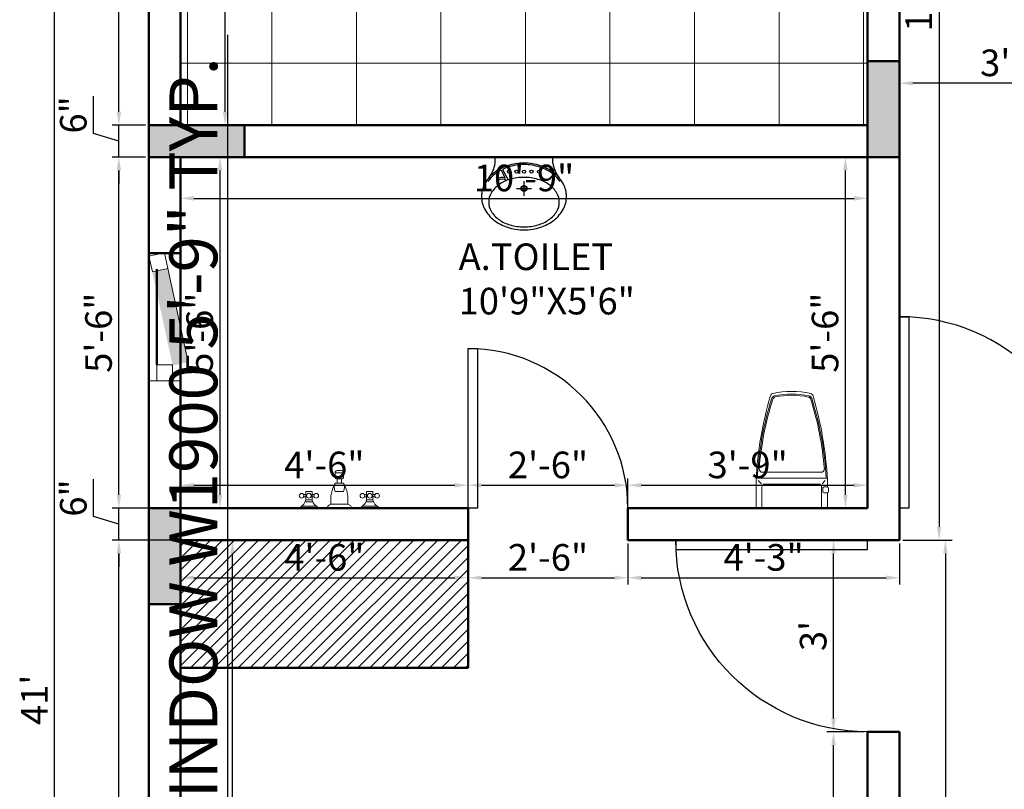
# Model space of a CAD drawing. Units: inches. Extents: x 3064 to 19385, y 846 to 15425.
# Tile 100 of 108: x 7502 to 7687, y 1134 to 1278. Entities that reach past the tile are written whole.
import ezdxf

# ---------------------------------------------------------------- set-up
doc = ezdxf.new("R2010")
doc.units = ezdxf.units.IN
for name, color, linetype, lineweight in [('A-ANNO-DIMS', 2, 'Continuous', 18), ('A-AREA-IDEN', 3, 'Continuous', 18), ('A-COLS', 1, 'Continuous', 35), ('A-DOOR', 3, 'Continuous', 25), ('A-FLOR-FIXT', 9, 'Continuous', 18), ('A-FLOR-PATT', 252, 'Continuous', 13), ('A-FURN-PATT', 252, 'Continuous', 13), ('A-GLAZ', 4, 'Continuous', 18), ('A-WALL', 7, 'Continuous', 50)]:
    doc.layers.add(name, color=color, linetype=linetype, lineweight=lineweight)
doc.layers.add('THIET-BI', color=21, linetype='Continuous')
doc.styles.get("Standard").update_dxf_attribs({"font": 'arial.ttf'})
doc.dimstyles.new('ISO-25', dxfattribs={"dimtxt": 9, "dimasz": 2.5, "dimexe": 1.25, "dimexo": 0.625, "dimtad": 1, "dimdec": 1, "dimlunit": 3, "dimtxsty": 'Standard', "dimcen": 2.5, "dimadec": 0, "dimazin": 0, "dimtfac": 1, "dimtdec": 1, "dimtmove": 0, "dimatfit": 3, "dimfxl": 1, "dimarcsym": 0})

# ---------------------------------------------------------------- blocks, each defined once
blk = doc.blocks.new('*U3')
for p, q in [((0, 0), (0, -6)), ((36, 0), (36, -6))]:
    blk.add_line(p, q)
blk.add_lwpolyline([(0, 0), (0, 36), (1.75, 36), (1.75, 0)], close=True)
blk.add_arc((0, 0), 36, 0, 90)
blk = doc.blocks.new('*U4')
for p, q in [((0, 0), (0, -6)), ((30, 0), (30, -6))]:
    blk.add_line(p, q)
blk.add_lwpolyline([(0, 0), (0, 30), (1.75, 30), (1.75, 0)], close=True)
blk.add_arc((0, 0), 30, 0, 90)
blk = doc.blocks.new('*D318')
at = {"layer": 'A-ANNO-DIMS', "color": 0, "lineweight": -2, "transparency": 16777216}
for p, q in [((7531.62, 1180.34), (7519.4, 1180.34)), ((7520.65, 984.84), (7520.65, 1177.84)), ((7531.62, 982.34), (7519.4, 982.34))]:
    blk.add_line(p, q, dxfattribs=at)
at = {"layer": 'A-ANNO-DIMS', "color": 0, "transparency": 16777216}
for points in [[(7520.23, 1177.84), (7521.06, 1177.84), (7520.65, 1180.34)], [(7520.23, 984.84), (7521.06, 984.84), (7520.65, 982.34)]]:
    blk.add_solid(points, dxfattribs=at)
at = {"layer": 'Defpoints', "color": 0, "transparency": 16777216}
for p in [(7520.65, 1180.34), (7532.25, 1180.34), (7532.25, 982.34)]:
    blk.add_point(p, dxfattribs=at)
at = {"layer": 'A-ANNO-DIMS', "color": 0, "transparency": 16777216, "insert": (7517.47, 1081.34), "char_height": 5, "attachment_point": 5, "rotation": 90}
blk.add_mtext('16\'-6"', dxfattribs=at)
blk = doc.blocks.new('*D319')
at = {"layer": 'A-ANNO-DIMS', "color": 0, "lineweight": -2, "transparency": 16777216}
for p, q in [((7515.91, 1184.76), (7515.91, 1191.79)), ((7520.65, 1188.84), (7520.65, 1191.34)), ((7531.62, 1186.34), (7519.4, 1186.34)), ((7520.65, 1180.34), (7520.65, 1186.34)), ((7520.65, 1180.34), (7520.65, 1186.34)), ((7520.65, 1183.34), (7515.91, 1184.76)), ((7531.62, 1180.34), (7519.4, 1180.34)), ((7520.65, 1177.84), (7520.65, 1175.34))]:
    blk.add_line(p, q, dxfattribs=at)
at = {"layer": 'A-ANNO-DIMS', "color": 0, "transparency": 16777216}
for points in [[(7520.23, 1188.84), (7521.06, 1188.84), (7520.65, 1186.34)], [(7520.23, 1177.84), (7521.06, 1177.84), (7520.65, 1180.34)]]:
    blk.add_solid(points, dxfattribs=at)
at = {"layer": 'Defpoints', "color": 0, "transparency": 16777216}
for p in [(7520.65, 1186.34), (7532.25, 1186.34), (7532.25, 1180.34)]:
    blk.add_point(p, dxfattribs=at)
at = {"layer": 'A-ANNO-DIMS', "color": 0, "transparency": 16777216, "insert": (7512.73, 1188.27), "char_height": 5, "attachment_point": 5, "rotation": 90}
blk.add_mtext('6"', dxfattribs=at)
blk = doc.blocks.new('*D320')
at = {"layer": 'A-ANNO-DIMS', "color": 0, "lineweight": -2, "transparency": 16777216}
for p, q in [((7525.62, 1252.34), (7519.4, 1252.34)), ((7520.65, 1188.84), (7520.65, 1249.84)), ((7531.62, 1186.34), (7519.4, 1186.34))]:
    blk.add_line(p, q, dxfattribs=at)
at = {"layer": 'A-ANNO-DIMS', "color": 0, "transparency": 16777216}
for points in [[(7520.23, 1249.84), (7521.06, 1249.84), (7520.65, 1252.34)], [(7520.23, 1188.84), (7521.06, 1188.84), (7520.65, 1186.34)]]:
    blk.add_solid(points, dxfattribs=at)
at = {"layer": 'Defpoints', "color": 0, "transparency": 16777216}
for p in [(7520.65, 1252.34), (7526.25, 1252.34), (7532.25, 1186.34)]:
    blk.add_point(p, dxfattribs=at)
at = {"layer": 'A-ANNO-DIMS', "color": 0, "transparency": 16777216, "insert": (7517.47, 1219.34), "char_height": 5, "attachment_point": 5, "rotation": 90}
blk.add_mtext('5\'-6"', dxfattribs=at)
blk = doc.blocks.new('*D321')
at = {"layer": 'A-ANNO-DIMS', "color": 0, "lineweight": -2, "transparency": 16777216}
for p, q in [((7515.91, 1256.76), (7515.91, 1263.79)), ((7520.65, 1260.84), (7520.65, 1263.34)), ((7525.62, 1258.34), (7519.4, 1258.34)), ((7520.65, 1252.34), (7520.65, 1258.34)), ((7520.65, 1252.34), (7520.65, 1258.34)), ((7520.65, 1255.34), (7515.91, 1256.76)), ((7525.62, 1252.34), (7519.4, 1252.34)), ((7520.65, 1249.84), (7520.65, 1247.34))]:
    blk.add_line(p, q, dxfattribs=at)
at = {"layer": 'A-ANNO-DIMS', "color": 0, "transparency": 16777216}
for points in [[(7520.23, 1260.84), (7521.06, 1260.84), (7520.65, 1258.34)], [(7520.23, 1249.84), (7521.06, 1249.84), (7520.65, 1252.34)]]:
    blk.add_solid(points, dxfattribs=at)
at = {"layer": 'Defpoints', "color": 0, "transparency": 16777216}
for p in [(7520.65, 1258.34), (7526.25, 1258.34), (7526.25, 1252.34)]:
    blk.add_point(p, dxfattribs=at)
at = {"layer": 'A-ANNO-DIMS', "color": 0, "transparency": 16777216, "insert": (7512.73, 1260.27), "char_height": 5, "attachment_point": 5, "rotation": 90}
blk.add_mtext('6"', dxfattribs=at)
blk = doc.blocks.new('*D322')
at = {"layer": 'A-ANNO-DIMS', "color": 0, "lineweight": -2, "transparency": 16777216}
for p, q in [((7531.62, 1390.34), (7519.4, 1390.34)), ((7520.65, 1260.84), (7520.65, 1387.84)), ((7525.62, 1258.34), (7519.4, 1258.34))]:
    blk.add_line(p, q, dxfattribs=at)
at = {"layer": 'A-ANNO-DIMS', "color": 0, "transparency": 16777216}
for points in [[(7520.23, 1387.84), (7521.06, 1387.84), (7520.65, 1390.34)], [(7520.23, 1260.84), (7521.06, 1260.84), (7520.65, 1258.34)]]:
    blk.add_solid(points, dxfattribs=at)
at = {"layer": 'Defpoints', "color": 0, "transparency": 16777216}
for p in [(7520.65, 1390.34), (7532.25, 1390.34), (7526.25, 1258.34)]:
    blk.add_point(p, dxfattribs=at)
at = {"layer": 'A-ANNO-DIMS', "color": 0, "transparency": 16777216, "insert": (7517.51, 1324.34), "char_height": 5, "attachment_point": 5, "rotation": 90}
blk.add_mtext("11'", dxfattribs=at)
blk = doc.blocks.new('*D324')
at = {"layer": 'A-ANNO-DIMS', "color": 0, "lineweight": -2, "transparency": 16777216}
for p, q in [((7525.62, 1396.34), (7507.31, 1396.34)), ((7508.56, 906.84), (7508.56, 1393.84)), ((7525.62, 904.34), (7507.31, 904.34))]:
    blk.add_line(p, q, dxfattribs=at)
at = {"layer": 'A-ANNO-DIMS', "color": 0, "transparency": 16777216}
for points in [[(7508.15, 1393.84), (7508.98, 1393.84), (7508.56, 1396.34)], [(7508.15, 906.84), (7508.98, 906.84), (7508.56, 904.34)]]:
    blk.add_solid(points, dxfattribs=at)
at = {"layer": 'Defpoints', "color": 0, "transparency": 16777216}
for p in [(7508.56, 1396.34), (7526.25, 1396.34), (7526.25, 904.34)]:
    blk.add_point(p, dxfattribs=at)
at = {"layer": 'A-ANNO-DIMS', "color": 0, "transparency": 16777216, "insert": (7505.43, 1150.34), "char_height": 5, "attachment_point": 5, "rotation": 90}
blk.add_mtext("41'", dxfattribs=at)
blk = doc.blocks.new('*D219')
at = {"layer": 'A-ANNO-DIMS', "color": 0, "lineweight": -2, "transparency": 16777216}
for p, q in [((7532.87, 1180.34), (7543.24, 1180.34)), ((7541.99, 984.84), (7541.99, 1177.84)), ((7532.87, 982.34), (7543.24, 982.34))]:
    blk.add_line(p, q, dxfattribs=at)
at = {"layer": 'A-ANNO-DIMS', "color": 0, "transparency": 16777216}
for points in [[(7541.58, 1177.84), (7542.41, 1177.84), (7541.99, 1180.34)], [(7541.58, 984.84), (7542.41, 984.84), (7541.99, 982.34)]]:
    blk.add_solid(points, dxfattribs=at)
at = {"layer": 'Defpoints', "color": 0, "transparency": 16777216}
for p in [(7532.25, 1180.34), (7541.99, 1180.34), (7532.25, 982.34)]:
    blk.add_point(p, dxfattribs=at)
at = {"layer": 'A-ANNO-DIMS', "color": 0, "transparency": 16777216, "insert": (7538.82, 1081.34), "char_height": 5, "attachment_point": 5, "rotation": 90}
blk.add_mtext('16\'-6"', dxfattribs=at)
blk = doc.blocks.new('*D263')
at = {"layer": 'A-ANNO-DIMS', "color": 0, "lineweight": -2, "transparency": 16777216}
for p, q in [((7532.25, 1179.71), (7532.25, 1172.03)), ((7586.25, 1179.71), (7586.25, 1172.03)), ((7534.75, 1173.28), (7583.75, 1173.28))]:
    blk.add_line(p, q, dxfattribs=at)
at = {"layer": 'A-ANNO-DIMS', "color": 0, "transparency": 16777216}
for points in [[(7534.75, 1173.7), (7534.75, 1172.87), (7532.25, 1173.28)], [(7583.75, 1173.7), (7583.75, 1172.87), (7586.25, 1173.28)]]:
    blk.add_solid(points, dxfattribs=at)
at = {"layer": 'Defpoints', "color": 0, "transparency": 16777216}
for p in [(7532.25, 1180.34), (7586.25, 1180.34), (7586.25, 1173.28)]:
    blk.add_point(p, dxfattribs=at)
at = {"layer": 'A-ANNO-DIMS', "color": 0, "transparency": 16777216, "insert": (7559.25, 1176.46), "char_height": 5, "attachment_point": 5}
blk.add_mtext('4\'-6"', dxfattribs=at)
blk = doc.blocks.new('*D232')
at = {"layer": 'A-ANNO-DIMS', "color": 0, "lineweight": -2, "transparency": 16777216}
for p, q in [((7586.25, 1179.71), (7586.25, 1172.03)), ((7616.25, 1179.71), (7616.25, 1172.03)), ((7588.75, 1173.28), (7613.75, 1173.28))]:
    blk.add_line(p, q, dxfattribs=at)
at = {"layer": 'A-ANNO-DIMS', "color": 0, "transparency": 16777216}
for points in [[(7588.75, 1173.7), (7588.75, 1172.87), (7586.25, 1173.28)], [(7613.75, 1173.7), (7613.75, 1172.87), (7616.25, 1173.28)]]:
    blk.add_solid(points, dxfattribs=at)
at = {"layer": 'Defpoints', "color": 0, "transparency": 16777216}
for p in [(7586.25, 1180.34), (7616.25, 1180.34), (7616.25, 1173.28)]:
    blk.add_point(p, dxfattribs=at)
at = {"layer": 'A-ANNO-DIMS', "color": 0, "transparency": 16777216, "insert": (7601.25, 1176.46), "char_height": 5, "attachment_point": 5}
blk.add_mtext('2\'-6"', dxfattribs=at)
blk = doc.blocks.new('*D233')
at = {"layer": 'A-ANNO-DIMS', "color": 0, "lineweight": -2, "transparency": 16777216}
for p, q in [((7616.25, 1179.71), (7616.25, 1172.03)), ((7667.25, 1179.71), (7667.25, 1172.03)), ((7618.75, 1173.28), (7664.75, 1173.28))]:
    blk.add_line(p, q, dxfattribs=at)
at = {"layer": 'A-ANNO-DIMS', "color": 0, "transparency": 16777216}
for points in [[(7618.75, 1173.7), (7618.75, 1172.87), (7616.25, 1173.28)], [(7664.75, 1173.7), (7664.75, 1172.87), (7667.25, 1173.28)]]:
    blk.add_solid(points, dxfattribs=at)
at = {"layer": 'Defpoints', "color": 0, "transparency": 16777216}
for p in [(7616.25, 1180.34), (7667.25, 1180.34), (7667.25, 1173.28)]:
    blk.add_point(p, dxfattribs=at)
at = {"layer": 'A-ANNO-DIMS', "color": 0, "transparency": 16777216, "insert": (7641.75, 1176.46), "char_height": 5, "attachment_point": 5}
blk.add_mtext('4\'-3"', dxfattribs=at)
blk = doc.blocks.new('*D234')
at = {"layer": 'A-ANNO-DIMS', "color": 0, "lineweight": -2, "transparency": 16777216}
for p, q in [((7660.62, 1144.34), (7653.63, 1144.34)), ((7654.88, 984.84), (7654.88, 1141.84)), ((7660.62, 982.34), (7653.63, 982.34))]:
    blk.add_line(p, q, dxfattribs=at)
at = {"layer": 'A-ANNO-DIMS', "color": 0, "transparency": 16777216}
for points in [[(7654.46, 1141.84), (7655.29, 1141.84), (7654.88, 1144.34)], [(7654.46, 984.84), (7655.29, 984.84), (7654.88, 982.34)]]:
    blk.add_solid(points, dxfattribs=at)
at = {"layer": 'Defpoints', "color": 0, "transparency": 16777216}
for p in [(7654.88, 1144.34), (7661.25, 1144.34), (7661.25, 982.34)]:
    blk.add_point(p, dxfattribs=at)
at = {"layer": 'A-ANNO-DIMS', "color": 0, "transparency": 16777216, "insert": (7651.7, 1063.34), "char_height": 5, "attachment_point": 5, "rotation": 90}
blk.add_mtext('13\'-6"', dxfattribs=at)
blk = doc.blocks.new('*D235')
at = {"layer": 'A-ANNO-DIMS', "color": 0, "lineweight": -2, "transparency": 16777216}
for p, q in [((7655.5, 1180.34), (7656.13, 1180.34)), ((7654.88, 1146.84), (7654.88, 1177.84)), ((7660.62, 1144.34), (7653.63, 1144.34))]:
    blk.add_line(p, q, dxfattribs=at)
at = {"layer": 'A-ANNO-DIMS', "color": 0, "transparency": 16777216}
for points in [[(7654.46, 1177.84), (7655.29, 1177.84), (7654.88, 1180.34)], [(7654.46, 1146.84), (7655.29, 1146.84), (7654.88, 1144.34)]]:
    blk.add_solid(points, dxfattribs=at)
at = {"layer": 'Defpoints', "color": 0, "transparency": 16777216}
for p in [(7654.88, 1180.34), (7654.88, 1180.34), (7661.25, 1144.34)]:
    blk.add_point(p, dxfattribs=at)
at = {"layer": 'A-ANNO-DIMS', "color": 0, "transparency": 16777216, "insert": (7651.7, 1162.34), "char_height": 5, "attachment_point": 5, "rotation": 90}
blk.add_mtext("3'", dxfattribs=at)
blk = doc.blocks.new('*D236')
at = {"layer": 'A-ANNO-DIMS', "color": 0, "lineweight": -2, "transparency": 16777216}
for p, q in [((7532.25, 1186.96), (7532.25, 1191.91)), ((7586.25, 1186.96), (7586.25, 1191.91)), ((7534.75, 1190.66), (7583.75, 1190.66))]:
    blk.add_line(p, q, dxfattribs=at)
at = {"layer": 'A-ANNO-DIMS', "color": 0, "transparency": 16777216}
for points in [[(7534.75, 1191.08), (7534.75, 1190.24), (7532.25, 1190.66)], [(7583.75, 1191.08), (7583.75, 1190.24), (7586.25, 1190.66)]]:
    blk.add_solid(points, dxfattribs=at)
at = {"layer": 'Defpoints', "color": 0, "transparency": 16777216}
for p in [(7586.25, 1190.66), (7532.25, 1186.34), (7586.25, 1186.34)]:
    blk.add_point(p, dxfattribs=at)
at = {"layer": 'A-ANNO-DIMS', "color": 0, "transparency": 16777216, "insert": (7559.25, 1193.84), "char_height": 5, "attachment_point": 5}
blk.add_mtext('4\'-6"', dxfattribs=at)
blk = doc.blocks.new('*D255')
at = {"layer": 'A-ANNO-DIMS', "color": 0, "lineweight": -2, "transparency": 16777216}
for p, q in [((7586.25, 1186.96), (7586.25, 1191.91)), ((7616.25, 1186.96), (7616.25, 1191.91)), ((7588.75, 1190.66), (7613.75, 1190.66))]:
    blk.add_line(p, q, dxfattribs=at)
at = {"layer": 'A-ANNO-DIMS', "color": 0, "transparency": 16777216}
for points in [[(7588.75, 1191.08), (7588.75, 1190.24), (7586.25, 1190.66)], [(7613.75, 1191.08), (7613.75, 1190.24), (7616.25, 1190.66)]]:
    blk.add_solid(points, dxfattribs=at)
at = {"layer": 'Defpoints', "color": 0, "transparency": 16777216}
for p in [(7616.25, 1190.66), (7586.25, 1186.34), (7616.25, 1186.34)]:
    blk.add_point(p, dxfattribs=at)
at = {"layer": 'A-ANNO-DIMS', "color": 0, "transparency": 16777216, "insert": (7601.25, 1193.84), "char_height": 5, "attachment_point": 5}
blk.add_mtext('2\'-6"', dxfattribs=at)
blk = doc.blocks.new('*D256')
at = {"layer": 'A-ANNO-DIMS', "color": 0, "lineweight": -2, "transparency": 16777216}
for p, q in [((7616.25, 1186.96), (7616.25, 1191.91)), ((7661.25, 1186.96), (7661.25, 1191.91)), ((7618.75, 1190.66), (7658.75, 1190.66))]:
    blk.add_line(p, q, dxfattribs=at)
at = {"layer": 'A-ANNO-DIMS', "color": 0, "transparency": 16777216}
for points in [[(7618.75, 1191.08), (7618.75, 1190.24), (7616.25, 1190.66)], [(7658.75, 1191.08), (7658.75, 1190.24), (7661.25, 1190.66)]]:
    blk.add_solid(points, dxfattribs=at)
at = {"layer": 'Defpoints', "color": 0, "transparency": 16777216}
for p in [(7661.25, 1190.66), (7616.25, 1186.34), (7661.25, 1186.34)]:
    blk.add_point(p, dxfattribs=at)
at = {"layer": 'A-ANNO-DIMS', "color": 0, "transparency": 16777216, "insert": (7638.75, 1193.84), "char_height": 5, "attachment_point": 5}
blk.add_mtext('3\'-9"', dxfattribs=at)
blk = doc.blocks.new('*D257')
at = {"layer": 'A-ANNO-DIMS', "color": 0, "lineweight": -2, "transparency": 16777216}
for p, q in [((7660.62, 1252.34), (7655.86, 1252.34)), ((7657.11, 1188.84), (7657.11, 1249.84)), ((7660.62, 1186.34), (7655.86, 1186.34))]:
    blk.add_line(p, q, dxfattribs=at)
at = {"layer": 'A-ANNO-DIMS', "color": 0, "transparency": 16777216}
for points in [[(7656.69, 1249.84), (7657.52, 1249.84), (7657.11, 1252.34)], [(7656.69, 1188.84), (7657.52, 1188.84), (7657.11, 1186.34)]]:
    blk.add_solid(points, dxfattribs=at)
at = {"layer": 'Defpoints', "color": 0, "transparency": 16777216}
for p in [(7657.11, 1252.34), (7661.25, 1252.34), (7661.25, 1186.34)]:
    blk.add_point(p, dxfattribs=at)
at = {"layer": 'A-ANNO-DIMS', "color": 0, "transparency": 16777216, "insert": (7653.93, 1219.34), "char_height": 5, "attachment_point": 5, "rotation": 90}
blk.add_mtext('5\'-6"', dxfattribs=at)
blk = doc.blocks.new('*D258')
at = {"layer": 'A-ANNO-DIMS', "color": 0, "lineweight": -2, "transparency": 16777216}
for p, q in [((7532.25, 1251.71), (7532.25, 1243.33)), ((7661.25, 1251.71), (7661.25, 1243.33)), ((7534.75, 1244.58), (7658.75, 1244.58))]:
    blk.add_line(p, q, dxfattribs=at)
at = {"layer": 'A-ANNO-DIMS', "color": 0, "transparency": 16777216}
for points in [[(7534.75, 1245), (7534.75, 1244.16), (7532.25, 1244.58)], [(7658.75, 1245), (7658.75, 1244.16), (7661.25, 1244.58)]]:
    blk.add_solid(points, dxfattribs=at)
at = {"layer": 'Defpoints', "color": 0, "transparency": 16777216}
for p in [(7532.25, 1252.34), (7661.25, 1252.34), (7661.25, 1244.58)]:
    blk.add_point(p, dxfattribs=at)
at = {"layer": 'A-ANNO-DIMS', "color": 0, "transparency": 16777216, "insert": (7596.75, 1247.76), "char_height": 5, "attachment_point": 5}
blk.add_mtext('10\'-9"', dxfattribs=at)
blk = doc.blocks.new('*D218')
at = {"layer": 'A-ANNO-DIMS', "color": 0, "lineweight": -2, "transparency": 16777216}
for p, q in [((7532.87, 1252.34), (7540.89, 1252.34)), ((7539.64, 1249.84), (7539.64, 1188.84)), ((7532.87, 1186.34), (7540.89, 1186.34))]:
    blk.add_line(p, q, dxfattribs=at)
at = {"layer": 'A-ANNO-DIMS', "color": 0, "transparency": 16777216}
for points in [[(7539.22, 1249.84), (7540.05, 1249.84), (7539.64, 1252.34)], [(7539.22, 1188.84), (7540.05, 1188.84), (7539.64, 1186.34)]]:
    blk.add_solid(points, dxfattribs=at)
at = {"layer": 'Defpoints', "color": 0, "transparency": 16777216}
for p in [(7532.25, 1252.34), (7532.25, 1186.34), (7539.64, 1186.34)]:
    blk.add_point(p, dxfattribs=at)
at = {"layer": 'A-ANNO-DIMS', "color": 0, "transparency": 16777216, "insert": (7536.46, 1219.34), "char_height": 5, "attachment_point": 5, "rotation": 90}
blk.add_mtext('5\'-6"', dxfattribs=at)
blk = doc.blocks.new('*D227')
at = {"layer": 'A-ANNO-DIMS', "color": 0, "lineweight": -2, "transparency": 16777216}
for p, q in [((7532.87, 1390.34), (7541.86, 1390.34)), ((7540.61, 1260.84), (7540.61, 1387.84)), ((7532.87, 1258.34), (7541.86, 1258.34))]:
    blk.add_line(p, q, dxfattribs=at)
at = {"layer": 'A-ANNO-DIMS', "color": 0, "transparency": 16777216}
for points in [[(7540.19, 1387.84), (7541.03, 1387.84), (7540.61, 1390.34)], [(7540.19, 1260.84), (7541.03, 1260.84), (7540.61, 1258.34)]]:
    blk.add_solid(points, dxfattribs=at)
at = {"layer": 'Defpoints', "color": 0, "transparency": 16777216}
for p in [(7532.25, 1390.34), (7540.61, 1390.34), (7532.25, 1258.34)]:
    blk.add_point(p, dxfattribs=at)
at = {"layer": 'A-ANNO-DIMS', "color": 0, "transparency": 16777216, "insert": (7537.48, 1324.34), "char_height": 5, "attachment_point": 5, "rotation": 90}
blk.add_mtext("11'", dxfattribs=at)
blk = doc.blocks.new('*D229')
at = {"layer": 'A-ANNO-DIMS', "color": 0, "lineweight": -2, "transparency": 16777216}
for p, q in [((7667.87, 1390.34), (7675.96, 1390.34)), ((7674.71, 1387.84), (7674.71, 1182.84)), ((7667.87, 1180.34), (7675.96, 1180.34))]:
    blk.add_line(p, q, dxfattribs=at)
at = {"layer": 'A-ANNO-DIMS', "color": 0, "transparency": 16777216}
for points in [[(7674.29, 1387.84), (7675.12, 1387.84), (7674.71, 1390.34)], [(7674.29, 1182.84), (7675.12, 1182.84), (7674.71, 1180.34)]]:
    blk.add_solid(points, dxfattribs=at)
at = {"layer": 'Defpoints', "color": 0, "transparency": 16777216}
for p in [(7667.25, 1390.34), (7667.25, 1180.34), (7674.71, 1180.34)]:
    blk.add_point(p, dxfattribs=at)
at = {"layer": 'A-ANNO-DIMS', "color": 0, "transparency": 16777216, "insert": (7671.53, 1285.34), "char_height": 5, "attachment_point": 5, "rotation": 90}
blk.add_mtext('17\'-6"', dxfattribs=at)
blk = doc.blocks.new('*D243')
at = {"layer": 'A-ANNO-DIMS', "color": 0, "lineweight": -2, "transparency": 16777216}
for p, q in [((7667.25, 1269.71), (7667.25, 1264.97)), ((7703.25, 1258.96), (7703.25, 1267.47)), ((7700.75, 1266.22), (7669.75, 1266.22))]:
    blk.add_line(p, q, dxfattribs=at)
at = {"layer": 'A-ANNO-DIMS', "color": 0, "transparency": 16777216}
for points in [[(7669.75, 1266.64), (7669.75, 1265.81), (7667.25, 1266.22)], [(7700.75, 1266.64), (7700.75, 1265.81), (7703.25, 1266.22)]]:
    blk.add_solid(points, dxfattribs=at)
at = {"layer": 'Defpoints', "color": 0, "transparency": 16777216}
for p in [(7667.25, 1270.34), (7667.25, 1266.22), (7703.25, 1258.34)]:
    blk.add_point(p, dxfattribs=at)
at = {"layer": 'A-ANNO-DIMS', "color": 0, "transparency": 16777216, "insert": (7685.25, 1269.4), "char_height": 5, "attachment_point": 5}
blk.add_mtext("3'", dxfattribs=at)
blk = doc.blocks.new('*D244')
at = {"layer": 'A-ANNO-DIMS', "color": 0, "lineweight": -2, "transparency": 16777216}
for p, q in [((7667.87, 1180.34), (7677.14, 1180.34)), ((7675.89, 1177.84), (7675.89, 984.84)), ((7667.87, 982.34), (7677.14, 982.34))]:
    blk.add_line(p, q, dxfattribs=at)
at = {"layer": 'A-ANNO-DIMS', "color": 0, "transparency": 16777216}
for points in [[(7675.47, 1177.84), (7676.3, 1177.84), (7675.89, 1180.34)], [(7675.47, 984.84), (7676.3, 984.84), (7675.89, 982.34)]]:
    blk.add_solid(points, dxfattribs=at)
at = {"layer": 'Defpoints', "color": 0, "transparency": 16777216}
for p in [(7667.25, 1180.34), (7667.25, 982.34), (7675.89, 982.34)]:
    blk.add_point(p, dxfattribs=at)
at = {"layer": 'A-ANNO-DIMS', "color": 0, "transparency": 16777216, "insert": (7672.71, 1081.34), "char_height": 5, "attachment_point": 5, "rotation": 90}
blk.add_mtext('16\'-6"', dxfattribs=at)
blk = doc.blocks.new('A$C430D11A0')
at = {"layer": 'THIET-BI'}
for p, q in [((90, 445), (90, 485)), ((475, 485), (90, 485)), ((475, 483), (90, 483)), ((475, 445), (475, 485)), ((129.4, 398.5), (158.2, 344.4)), ((138.3, 403), (176, 332.4)), ((233.4, 275.5), (331.9, 275.5)), ((282.5, 226.2), (282.5, 324.8))]:
    blk.add_line(p, q, dxfattribs=at)
for points in [[(565, 222.5, 0.121635), (544.7, 304.8, 0.10526), (482.3, 379.8, 0.088175), (393.4, 427.4, 0.079002), (282.5, 445, 0.079002), (171.6, 427.4, 0.088175), (82.7, 379.8, 0.10526), (20.3, 304.8, 0.121635), (0, 222.5, 0.121635), (20.3, 140.2, 0.10526), (82.7, 65.2, 0.088175), (171.6, 17.6, 0.079002), (282.5, 0, 0.079002), (393.4, 17.6, 0.088175), (482.3, 65.2, 0.10526), (544.7, 140.2, 0.121635)], [(517.5, 185, 0.134042), (501.2, 244.9, 0.106817), (448.7, 301.7, 0.082468), (375.6, 336.7, 0.070874), (282.5, 350, 0.070874), (189.4, 336.7, 0.082468), (116.3, 301.7, 0.106817), (63.8, 244.9, 0.134042), (47.5, 185, 0.134042), (63.8, 125.1, 0.106817), (116.3, 68.3, 0.082468), (189.4, 33.3, 0.070874), (282.5, 20, 0.070874), (375.6, 33.3, 0.082468), (448.7, 68.3, 0.106817), (501.2, 125.1, 0.134042)]]:
    blk.add_lwpolyline(points, format="xyb", close=True, dxfattribs=at)
for points in [[(129.4, 398.5, 0.043566), (88.9, 372, 0.07708), (42.1, 321.6, 0.041486)], [(522.9, 321.6, 0.07708), (476.1, 372, 0.088175), (390.3, 417.9, 0.079002), (282.5, 435, 0.079002), (174.7, 417.9, 0.035427), (138.3, 403, 0.07708)]]:
    blk.add_lwpolyline(points, format="xyb", dxfattribs=at)
for centre, radius in [((182.5, 388.2), 10.5), ((232.5, 388.2), 10.5), ((282.5, 388.2), 10.5), ((332.5, 388.2), 10.5), ((382.5, 388.2), 10.5), ((282.5, 275.5), 20), ((282.5, 275.5), 15)]:
    blk.add_circle(centre, radius, dxfattribs=at)
for centre, radius, start, end in [((-103.8, 468.9), 195.3, 320.8253, 352.95569), ((668.8, 468.9), 195.3, 187.04431, 219.1747), ((136.4, 285.4), 62.9, 69.64296, 123.47738), ((136.4, 285.4), 52.9, 55.24551, 123.47738)]:
    blk.add_arc(centre, radius, start, end, dxfattribs=at)
blk = doc.blocks.new('WC-P05')
for p, q in [((-202.4, 531.6), (-202.4, 439.1)), ((-192.4, 541.6), (262.6, 541.6)), ((-163.4, 541.6), (-163.4, 400.6)), ((233.6, 541.6), (233.6, 400.6)), ((272.6, 531.6), (272.6, 351.6)), ((-210.4, 430.1), (-210.4, 409.1)), ((-202.4, 400.1), (-202.4, 351.6)), ((-201.4, 439.1), (-180.4, 439.1)), ((-201.4, 400.1), (-180.4, 400.1)), ((-171.4, 430.1), (-171.4, 409.1)), ((-192.4, 341.6), (262.6, 341.6)), ((-166.9, 378.6), (-188.2, 357.3)), ((-143.4, 380.6), (213.6, 380.6)), ((237.1, 378.6), (258.4, 357.3)), ((-159.3, 302.6), (229.5, 302.6))]:
    blk.add_line(p, q)
blk.add_lwpolyline([(-90.9, -221.9, 0.114547), (161, -222, 0.114547)], format="xyb")
for centre, radius, start, end in [((-192.4, 531.6), 10, 90, 180), ((262.6, 531.6), 10, 0, 90), ((-201.4, 430.1), 9, 90, 180), ((-201.4, 409.1), 9, 180, 270), ((-180.4, 430.1), 9, 0, 90), ((-180.4, 409.1), 9, 270, 0), ((-143.4, 400.6), 20, 180, 270), ((213.6, 400.6), 20, 270, 0), ((2308.9, 492.3), 2515.2, 183.20675, 196.12415), ((-192.4, 351.6), 10, 180, 270), ((1906, 447.2), 2102.6, 182.87428, 197.65536), ((-1835.8, 447.2), 2102.6, 342.34464, 357.12572), ((-2238.7, 492.3), 2515.2, 343.87268, 356.79325), ((262.6, 351.6), 10, 270, 0), ((-159.3, 280.1), 22.5, 90, 184.62462), ((1905.9, 447.2), 2094.5, 184.62454, 197.52765), ((-1835.8, 447.2), 2094.6, 342.46396, 355.37538), ((229.5, 280.1), 22.5, 355.37538, 90), ((-76.1, -183.7), 22.5, 197.65536, 257.50587), ((-69.9, -176.8), 22.5, 197.52765, 258.10049), ((139.9, -177.1), 22.5, 281.73735, 342.46396), ((146.2, -183.7), 22.5, 282.49413, 342.34464), ((-85.8, -199.9), 22.5, 196.12415, 256.89941), ((35.1, 318), 536.4, 257.50587, 282.49413), ((35.7, 324.3), 534.7, 258.10049, 281.73735), ((155.9, -200.1), 22.5, 283.03778, 343.87268)]:
    blk.add_arc(centre, radius, start, end)
blk = doc.blocks.new('Faucet - Bathroom front')
for p, q in [((-0.5, 4.25), (0.5, 4.25)), ((0.5, 3.75), (-0.5, 3.75)), ((-0.5, 3), (0.5, 3)), ((-0.25, 3), (-0.25, 3.5)), ((0.25, 3.5), (0.25, 3)), ((-4, 1.625), (-4.25, 1.625)), ((-4, 1.375), (-4.25, 1.375)), ((-3.25, 1.625), (-3, 1.625)), ((-3.25, 1.375), (-3, 1.375)), ((0.5, 2), (-0.5, 2)), ((3.25, 1.625), (3, 1.625)), ((3.25, 1.375), (3, 1.375)), ((4, 1.625), (4.25, 1.625)), ((4, 1.375), (4.25, 1.375)), ((-5, 0), (-2.25, 0)), ((-4.5087, 0.25), (-2.7408, 0.25)), ((-3.1442, 0.75), (-4.0979, 0.75)), ((-1.5, 0), (1.5, 0)), ((-1, 0.5), (1, 0.5)), ((2.25, 0), (5, 0)), ((2.7413, 0.25), (4.5092, 0.25)), ((4.1058, 0.75), (3.1521, 0.75))]:
    blk.add_line(p, q)
for points in [[(-0.5, 3.75), (-0.5, 4.25)], [(-0.25, 4.5), (0.25, 4.5)], [(0.5, 4.25), (0.5, 3.75)], [(0.25, 3.5), (-0.25, 3.5)]]:
    blk.add_lwpolyline(points)
for points in [[(-4, 1), (-4, 2), (-3.25, 2), (-3.25, 1)], [(3.25, 1), (3.25, 2), (4, 2), (4, 1)]]:
    blk.add_lwpolyline(points, close=True)
for centre in [(-4.5, 1.5), (-3.625, 1.5), (-2.75, 1.5), (2.75, 1.5), (3.625, 1.5), (4.5, 1.5)]:
    blk.add_circle(centre, 0.2795)
for centre, radius, start, end in [((-0.2575, 4.2575), 0.2426, 88.22243, 181.7776), ((-0.2575, 3.7425), 0.2426, 178.2224, 271.7776), ((0.2575, 4.2575), 0.2426, 358.2224, 91.77757), ((0.2575, 3.7425), 0.2426, 268.2224, 1.777565), ((3, 1), 4.0311, 150.2551, 187.125), ((0.6413, 2.5), 1.246, 156.3417, 203.6583), ((-3, 1), 4.0311, 352.875, 29.74488), ((-0.6413, 2.5), 1.246, 336.3417, 23.65835), ((-5.375, 1.375), 1.4252, 285.2551, 344.7449), ((-1.875, 1.375), 1.4252, 195.2551, 254.7449), ((-0.7962, -0.2038), 0.7327, 106.1502, 163.8498), ((0.7962, -0.2038), 0.7327, 16.1502, 73.84979), ((1.875, 1.375), 1.4252, 285.2551, 344.7449), ((5.375, 1.375), 1.4252, 195.2551, 254.7449)]:
    blk.add_arc(centre, radius, start, end)
blk = doc.blocks.new('WIN-600')
h = blk.add_hatch(color=256)
h.dxf.hatch_style = 1
h.paths.add_polyline_path([(3, 18), (0, 18), (0, 0), (3, 0)])
blk.add_line((3, 18), (3, 0))
blk.add_lwpolyline([(3, 18), (0, 18), (0, 21), (3, 21)], close=True)
blk = doc.blocks.new('*D431')
at = {"layer": 'A-ANNO-DIMS', "color": 0, "lineweight": -2, "transparency": 16777216}
for p, q in [((7541.1, 1114.34), (7541.1, 1275.31)), ((7531.37, 1114.34), (7542.35, 1114.34)), ((7541.1, 1047.84), (7541.1, 1111.84)), ((7531.37, 1045.34), (7542.35, 1045.34))]:
    blk.add_line(p, q, dxfattribs=at)
at = {"layer": 'A-ANNO-DIMS', "color": 0, "transparency": 16777216}
for points in [[(7540.68, 1111.84), (7541.51, 1111.84), (7541.1, 1114.34)], [(7540.68, 1047.84), (7541.51, 1047.84), (7541.1, 1045.34)]]:
    blk.add_solid(points, dxfattribs=at)
at = {"layer": 'Defpoints', "color": 0, "transparency": 16777216}
for p in [(7530.75, 1114.34), (7541.1, 1114.34), (7530.75, 1045.34)]:
    blk.add_point(p, dxfattribs=at)
at = {"layer": 'A-ANNO-DIMS', "color": 0, "transparency": 16777216, "insert": (7535.81, 1196.07), "char_height": 9, "attachment_point": 5, "rotation": 90}
blk.add_mtext('WINDOW W1900 5\'-9" TYP.', dxfattribs=at)

msp = doc.modelspace()

# ---------------------------------------------------------------- hatches: boundary and pattern name
at = {"layer": 'A-COLS'}
h = msp.add_hatch(color=256, dxfattribs=at)
h.dxf.hatch_style = 1
h.paths.add_polyline_path([(7661.25, 1252.34), (7667.25, 1252.34), (7667.25, 1270.34), (7661.25, 1270.34)])
h = msp.add_hatch(color=256, dxfattribs=at)
h.dxf.hatch_style = 1
h.paths.add_polyline_path([(7544.25, 1252.34), (7544.25, 1258.34), (7526.25, 1258.34), (7526.25, 1252.34)])
h = msp.add_hatch(color=256, dxfattribs=at)
h.dxf.hatch_style = 1
h.paths.add_polyline_path([(7526.25, 1168.34), (7532.25, 1168.34), (7532.25, 1186.34), (7526.25, 1186.34)])
at = {"layer": 'A-FLOR-PATT'}
h = msp.add_hatch(dxfattribs=at)
h.set_pattern_fill('ANSI37', color=256, scale=5, angle=45)
h.set_pattern_definition([(90, (3183.753, 0), (-15.875, 0), []), (180, (3183.753, 0), (-2e-15, -15.875), [])])
h.paths.add_polyline_path([(7532.25, 1390.34), (7532.25, 1378.34), (7532.25, 1258.34), (7661.25, 1258.34), (7661.25, 1270.34), (7661.25, 1390.34)])
at = {"layer": 'A-FURN-PATT'}
h = msp.add_hatch(dxfattribs=at)
h.set_pattern_fill('ANSI31', color=256, scale=0.5)
h.set_pattern_definition([(45, (3183.7531, -6), (-1.122532, 1.122532), [])])
h.paths.add_polyline_path([(7586.25, 1180.34), (7532.25, 1180.34), (7532.25, 1162.34), (7532.25, 1156.34), (7586.25, 1156.34)])

# ---------------------------------------------------------------- linework, layer by layer
at = {"layer": 'A-GLAZ'}
msp.add_line((7526.25, 1210.28), (7532.25, 1210.28), dxfattribs=at)
msp.add_lwpolyline([(7530.75, 1210.28), (7527.75, 1210.28), (7527.75, 1213.28), (7530.75, 1213.28)], close=True, dxfattribs=at)
at = {"layer": 'A-WALL'}
for p, q in [((7526.25, 1396.34), (7526.25, 976.34)), ((7532.25, 1390.34), (7532.25, 1258.34)), ((7661.25, 1390.34), (7661.25, 1258.34)), ((7667.25, 1390.34), (7667.25, 1180.34)), ((7532.25, 1258.34), (7661.25, 1258.34)), ((7532.25, 1252.34), (7532.25, 1186.34)), ((7532.25, 1252.34), (7661.25, 1252.34)), ((7667.25, 1252.34), (7661.25, 1252.34)), ((7661.25, 1252.34), (7661.25, 1186.34)), ((7526.25, 1234.28), (7532.25, 1234.28)), ((7527.75, 1231.28), (7527.75, 1213.28)), ((7532.25, 1186.34), (7586.25, 1186.34)), ((7586.25, 1186.34), (7586.25, 1180.34)), ((7586.25, 1186.34), (7586.25, 1156.34)), ((7616.25, 1186.34), (7661.25, 1186.34)), ((7616.25, 1186.34), (7616.25, 1180.34)), ((7532.25, 1180.34), (7532.25, 982.34)), ((7532.25, 1180.34), (7586.25, 1180.34)), ((7616.25, 1180.34), (7667.25, 1180.34)), ((7532.25, 1156.34), (7586.25, 1156.34)), ((7661.25, 1144.34), (7661.25, 982.34)), ((7661.25, 1144.34), (7667.25, 1144.34)), ((7667.25, 1144.34), (7667.25, 976.34))]:
    msp.add_line(p, q, dxfattribs=at)
for points in [[(7667.25, 1252.34), (7667.25, 1270.34), (7661.25, 1270.34), (7661.25, 1252.34)], [(7544.25, 1258.34), (7526.25, 1258.34), (7526.25, 1252.34), (7544.25, 1252.34)], [(7532.25, 1168.34), (7532.25, 1186.34), (7526.25, 1186.34), (7526.25, 1168.34)]]:
    msp.add_lwpolyline(points, close=True, dxfattribs=at)

# ---------------------------------------------------------------- block references
at = {"layer": 'A-DOOR'}
for name, p in [('*U3', (7667.25, 1186.34)), ('*U4', (7586.25, 1186.34))]:
    msp.add_blockref(name, p, dxfattribs=at)
at = {"layer": 'A-DOOR', "xscale": -1, "rotation": 90}
msp.add_blockref('*U3', (7661.25, 1180.34), dxfattribs=at)
at = {"layer": 'A-FLOR-FIXT'}
for name, p, xscale, yscale, zscale in [('A$C430D11A0', (7588.77, 1238.65), 0.0282220760332506, 0.0282220760332506, 0.0282220760332506), ('Faucet - Bathroom front', (7562.06, 1186.34), 1.573166238287219, 1.573166238287219, 1.573166238287219)]:
    msp.add_blockref(name, p, dxfattribs=dict(at, xscale=xscale, yscale=yscale, zscale=zscale))
at = {"layer": 'A-FLOR-FIXT', "xscale": 0.0282220760332506, "yscale": 0.0282220760332506, "zscale": 0.0282220760332506, "rotation": 180}
msp.add_blockref('WC-P05', (7648.02, 1201.63), dxfattribs=at)
at = {"layer": 'A-GLAZ', "rotation": 12.21571913413091}
msp.add_blockref('WIN-600', (7530.75, 1213.17), dxfattribs=at)

# ---------------------------------------------------------------- texts
at = {"layer": 'A-AREA-IDEN', "insert": (7584.47, 1236.1), "char_height": 5, "attachment_point": 1}
msp.add_mtext_dynamic_manual_height_columns('A.TOILET\\P10\'9"X5\'6"', width=67.5924, gutter_width=12.5, heights=[0], dxfattribs=at)

# ---------------------------------------------------------------- dimensions: what is measured, and where the dimension line sits
at = {"layer": 'A-ANNO-DIMS'}
for base, p1, p2, override, picture, middle in [((7508.56, 1396.34), (7526.25, 904.34), (7526.25, 1396.34), {"dimtxt": 5, "dimclrd": 0, "dimclre": 0, "dimclrt": 0}, '*D324', (7505.43, 1150.34)), ((7520.65, 1390.34), (7526.25, 1258.34), (7532.25, 1390.34), {"dimtxt": 5, "dimclrd": 0, "dimclre": 0, "dimclrt": 0, "dimtmove": 1}, '*D322', (7517.51, 1324.34)), ((7540.61, 1390.34), (7532.25, 1258.34), (7532.25, 1390.34), {"dimtxt": 5, "dimclrd": 0, "dimclre": 0, "dimclrt": 0}, '*D227', (7537.48, 1324.34)), ((7674.71, 1180.34), (7667.25, 1390.34), (7667.25, 1180.34), {"dimtxt": 5, "dimclrd": 0, "dimclre": 0, "dimclrt": 0}, '*D229', (7671.53, 1285.34)), ((7520.65, 1258.34), (7526.25, 1252.34), (7526.25, 1258.34), {"dimtxt": 5, "dimclrd": 0, "dimclre": 0, "dimclrt": 0, "dimtmove": 1}, '*D321', (7512.73, 1257.39)), ((7520.65, 1252.34), (7532.25, 1186.34), (7526.25, 1252.34), {"dimtxt": 5, "dimclrd": 0, "dimclre": 0, "dimclrt": 0, "dimtmove": 1}, '*D320', (7517.47, 1219.34)), ((7539.64, 1186.34), (7532.25, 1252.34), (7532.25, 1186.34), {"dimtxt": 5, "dimclrd": 0, "dimclre": 0, "dimclrt": 0}, '*D218', (7536.46, 1219.34)), ((7657.11, 1252.34), (7661.25, 1186.34), (7661.25, 1252.34), {"dimtxt": 5, "dimclrd": 0, "dimclre": 0, "dimclrt": 0}, '*D257', (7653.93, 1219.34)), ((7520.65, 1186.34), (7532.25, 1180.34), (7532.25, 1186.34), {"dimtxt": 5, "dimclrd": 0, "dimclre": 0, "dimclrt": 0, "dimtmove": 1}, '*D319', (7512.73, 1185.39)), ((7520.65, 1180.34), (7532.25, 982.34), (7532.25, 1180.34), {"dimtxt": 5, "dimclrd": 0, "dimclre": 0, "dimclrt": 0, "dimtmove": 1}, '*D318', (7517.47, 1081.34)), ((7541.99, 1180.34), (7532.25, 982.34), (7532.25, 1180.34), {"dimtxt": 5, "dimclrd": 0, "dimclre": 0, "dimclrt": 0}, '*D219', (7538.82, 1081.34)), ((7654.88, 1180.34), (7661.25, 1144.34), (7654.88, 1180.34), {"dimtxt": 5, "dimclrd": 0, "dimclre": 0, "dimclrt": 0, "dimtmove": 1}, '*D235', (7651.7, 1162.34)), ((7675.89, 982.34), (7667.25, 1180.34), (7667.25, 982.34), {"dimtxt": 5, "dimclrd": 0, "dimclre": 0, "dimclrt": 0}, '*D244', (7672.71, 1081.34)), ((7654.88, 1144.34), (7661.25, 982.34), (7661.25, 1144.34), {"dimtxt": 5, "dimclrd": 0, "dimclre": 0, "dimclrt": 0}, '*D234', (7651.7, 1063.34))]:
    dim = msp.add_linear_dim(base=base, p1=p1, p2=p2, angle=90, dimstyle='ISO-25', override=override, dxfattribs=at)
    dim.commit()
    dim.dimension.update_dxf_attribs({"geometry": picture, "text_midpoint": middle})
dim = msp.add_linear_dim(base=(7541.1, 1114.34), p1=(7530.75, 1045.34), p2=(7530.75, 1114.34), angle=90, text='WINDOW W1900 <> TYP.', dimstyle='ISO-25', override={"dimdec": 1, "dimrnd": 0, "dimzin": 1, "dimlunit": 4, "dimfrac": 2}, dxfattribs=at)
dim.commit()
dim.dimension.update_dxf_attribs({"geometry": '*D431', "text_midpoint": (7535.81, 1196.07)})
for base, p1, p2, override, picture, middle in [((7667.25, 1266.22), (7703.25, 1258.34), (7667.25, 1270.34), {"dimtxt": 5, "dimclrd": 0, "dimclre": 0, "dimclrt": 0, "dimtmove": 1}, '*D243', (7685.25, 1269.4)), ((7661.25, 1244.58), (7532.25, 1252.34), (7661.25, 1252.34), {"dimtxt": 5, "dimclrd": 0, "dimclre": 0, "dimclrt": 0}, '*D258', (7596.75, 1247.76)), ((7586.25, 1190.66), (7532.25, 1186.34), (7586.25, 1186.34), {"dimtxt": 5, "dimclrd": 0, "dimclre": 0, "dimclrt": 0}, '*D236', (7559.25, 1193.84)), ((7616.25, 1190.66), (7586.25, 1186.34), (7616.25, 1186.34), {"dimtxt": 5, "dimclrd": 0, "dimclre": 0, "dimclrt": 0, "dimtmove": 1}, '*D255', (7601.25, 1193.84)), ((7661.25, 1190.66), (7616.25, 1186.34), (7661.25, 1186.34), {"dimtxt": 5, "dimclrd": 0, "dimclre": 0, "dimclrt": 0, "dimtmove": 1}, '*D256', (7638.75, 1193.84)), ((7586.25, 1173.28), (7532.25, 1180.34), (7586.25, 1180.34), {"dimtxt": 5, "dimclrd": 0, "dimclre": 0, "dimclrt": 0}, '*D263', (7559.25, 1176.46)), ((7616.25, 1173.28), (7586.25, 1180.34), (7616.25, 1180.34), {"dimtxt": 5, "dimclrd": 0, "dimclre": 0, "dimclrt": 0, "dimtmove": 1}, '*D232', (7601.25, 1176.46)), ((7667.25, 1173.28), (7616.25, 1180.34), (7667.25, 1180.34), {"dimtxt": 5, "dimclrd": 0, "dimclre": 0, "dimclrt": 0, "dimtmove": 1}, '*D233', (7641.75, 1176.46))]:
    dim = msp.add_linear_dim(base=base, p1=p1, p2=p2, dimstyle='ISO-25', override=override, dxfattribs=at)
    dim.commit()
    dim.dimension.update_dxf_attribs({"geometry": picture, "text_midpoint": middle})

doc.saveas('drawing.dxf')
